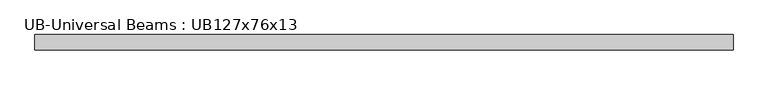
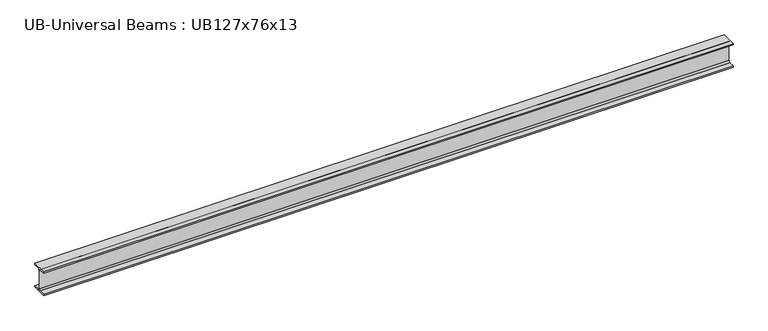
"""IFC4 building model written with IfcOpenShell, lengths in millimetres: member geometry, UB-Universal Beams : UB127x76x13."""

from ifc_helpers import new_model, si_unit, point, frame, frame_2d, origin, place, context, project, spatial, polyline, circle_curve, trimmed, segment, composite_curve, outline, extrude, source, transform, mapped, element, save


def ub_universal_beams_ub127x76x13_96cbbb94(model_context):
    return source(origin(), model_context, "Body", "SweptSolid", [
        extrude(outline(composite_curve([segment(polyline([(38.0, -55.9), (38.0, -63.5), (-38.0, -63.5), (-38.0, -55.9), (-9.6, -55.9)]), True, "CONTINUOUS"), segment(trimmed(circle_curve(frame_2d((-9.6, -48.3)), 7.6), [point((-9.6, -55.9))], [point((-2.0, -48.3))], True, "CARTESIAN"), True, "CONTINUOUS"), segment(polyline([(-2.0, -48.3), (-2.0, 48.3)]), True, "CONTINUOUS"), segment(trimmed(circle_curve(frame_2d((-9.6, 48.3)), 7.6), [point((-2.0, 48.3))], [point((-9.6, 55.9))], True, "CARTESIAN"), True, "CONTINUOUS"), segment(polyline([(-9.6, 55.9), (-38.0, 55.9), (-38.0, 63.5), (38.0, 63.5), (38.0, 55.9), (9.6, 55.9)]), True, "CONTINUOUS"), segment(trimmed(circle_curve(frame_2d((9.6, 48.3)), 7.6), [point((9.6, 55.9))], [point((2.0, 48.3))], True, "CARTESIAN"), True, "CONTINUOUS"), segment(polyline([(2.0, 48.3), (2.0, -48.3)]), True, "CONTINUOUS"), segment(trimmed(circle_curve(frame_2d((9.6, -48.3)), 7.6), [point((2.0, -48.3))], [point((9.6, -55.9))], True, "CARTESIAN"), True, "CONTINUOUS"), segment(polyline([(9.6, -55.9), (38.0, -55.9)]), True, "CONTINUOUS")], self_intersect=False)), frame((-1537.65, 0.0, 0.0), z_axis=(1.0, 0.0, 0.0), x_axis=(0.0, 1.0, 0.0)), (0.0, 0.0, 1.0), 3488.7),
    ])


if __name__ == "__main__":
    model = new_model("IFC4")
    model_context = context("Model", 3, world=origin())
    ifc_project = project(units=[si_unit("LENGTHUNIT", "METRE", prefix="MILLI")], contexts=[model_context])
    site = spatial("IfcSite", under=ifc_project)
    building = spatial("IfcBuilding", under=site)
    placement = place(None, origin())
    ub_universal_beams_ub127x76x13_shape = ub_universal_beams_ub127x76x13_96cbbb94(model_context)
    element("IfcMember", 1, ObjectType="UB-Universal Beams : UB127x76x13", at=placement, inside=building, context=model_context, shape_type="MappedRepresentation", body=[
        mapped(ub_universal_beams_ub127x76x13_shape, transform((0.0, 0.0, 0.0), x_axis=(1.0, 0.0, 0.0), y_axis=(0.0, 1.0, 0.0), z_axis=(0.0, 0.0, 1.0))),
    ])
    save(model, "model.ifc")

# Revit data of these elements
# Type "UB-Universal Beams : UB127x76x13"
#   Section Name Key = "UB127X76X13"
#   Width = 7.6 cm
#   Web Thickness = 0.4 cm
#   Web Fillet = 0.76 cm
#   Warping Constant = 2000.0 cm⁶
#   Torsional Moment of Inertia = 2.85 cm⁴
#   Section Area = 16.5 cm²
#   Plastic Modulus weak axis = 22.6 cm³
#   Plastic Modulus strong axis = 84.2 cm³
#   Nominal Weight = 13.00 kgf/m
#   Moment of Inertia weak axis = 55.70 cm⁴
#   Moment of Inertia strong axis = 473.00 cm⁴
#   Height = 12.7 cm
#   Flange Thickness = 0.76 cm
#   Elastic Modulus weak axis = 14.7 cm³
#   Elastic Modulus strong axis = 74.6 cm³
#   Centroid Vertical = 6.35 cm
#   Centroid Horizontal = 3.8 cm
#   Bolt Spacing = 4.0 cm
#   Length [instance default] = 1.5 m
#   Structural Material [instance default] = Metal - Steel 43-275
#   Type Comments = ""
#   Assembly Code = ""
# Element 1 (IfcMember, "UB-Universal Beams : UB127x76x13")
#   Materials on its faces: "Metal - Steel 43-275"
# Materials
#   "Metal - Steel 43-275": class "Metal", colour RGB 247 247 247, transparency 0, Cost = 0
